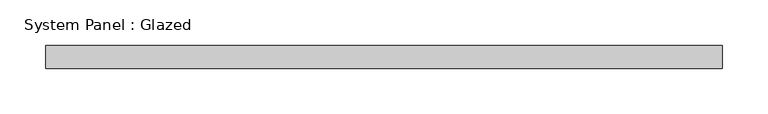
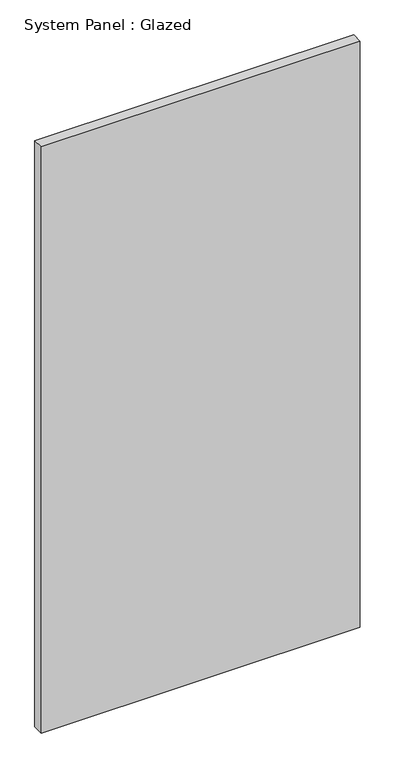
"""IFC4 building model written with IfcOpenShell, lengths in millimetres: plate geometry, System Panel : Glazed."""

from ifc_helpers import new_model, si_unit, origin, origin_with_axes, place, context, project, spatial, polyline, outline, extrude, source, transform, mapped, element, save


def system_panel_glazed_bfe2972e(model_context):
    return source(origin(), model_context, "Body", "SweptSolid", [
        extrude(outline(polyline([(371.475, 19.05), (-371.475, 19.05), (-371.475, 44.45), (371.475, 44.45), (371.475, 19.05)])), origin_with_axes(), (0.0, 0.0, 1.0), 1442.5186051),
    ])


if __name__ == "__main__":
    model = new_model("IFC4")
    model_context = context("Model", 3, world=origin())
    ifc_project = project(units=[si_unit("LENGTHUNIT", "METRE", prefix="MILLI")], contexts=[model_context])
    site = spatial("IfcSite", under=ifc_project)
    building = spatial("IfcBuilding", under=site)
    placement = place(None, origin())
    system_panel_glazed_shape = system_panel_glazed_bfe2972e(model_context)
    element("IfcPlate", 1, ObjectType="System Panel : Glazed", at=placement, inside=building, context=model_context, shape_type="MappedRepresentation", body=[
        mapped(system_panel_glazed_shape, transform((0.0, 0.0, 0.0), x_axis=(1.0, 0.0, 0.0), y_axis=(0.0, 1.0, 0.0), z_axis=(0.0, 0.0, 1.0))),
    ])
    save(model, "model.ifc")

# Revit data of these elements
# Type "System Panel : Glazed"
#   Construction Type Id = "GSP4R"
#   Analytic Construction = "1/8 in Pilkington single glazing"
#   Visual Light Transmittance = 0.9
#   Solar Heat Gain Coefficient = 0.86
#   Heat Transfer Coefficient (U) = 1.18115 BTU/(h·ft²·°F)
#   Define Thermal Properties by = 1
# Element 1 (IfcPlate, "System Panel : Glazed")
#   Materials on its faces: "Glass"
# Materials
#   "Glass": class "Glass", colour RGB 0 128 192, transparency 0.75, Description = "Soda Lime Glass", Cost = 0
